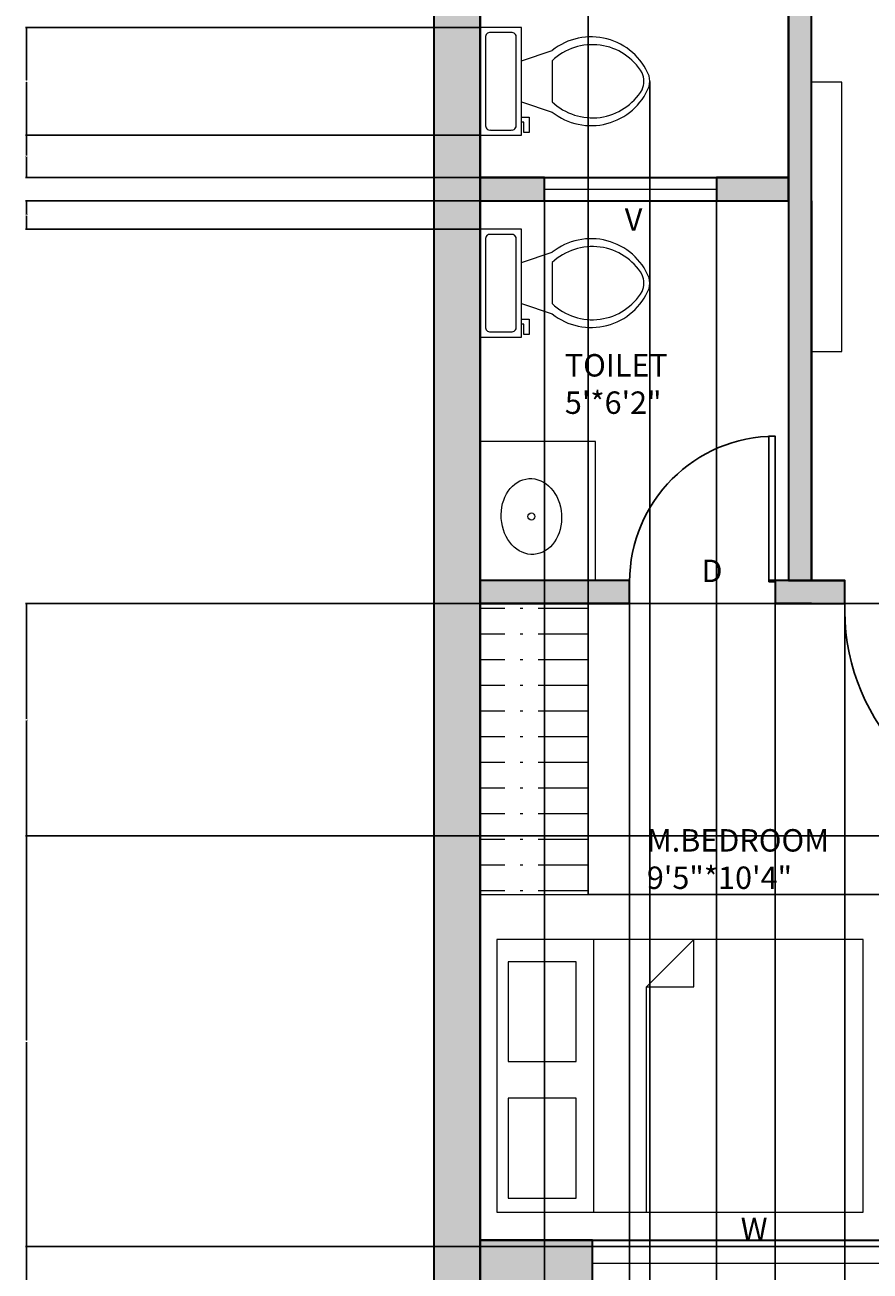
# Model space of a CAD drawing. Units: inches. Extents: x 2035 to 2384, y 1427 to 2020.
# Tile 2 of 7: x 2035 to 2200, y 1551 to 1794. Entities that reach past the tile are written whole.
import ezdxf

# ---------------------------------------------------------------- set-up
doc = ezdxf.new("R2010")
doc.units = ezdxf.units.IN
for name, color, linetype, lineweight in [('A-ANNO-DIMS', 2, 'Continuous', 18), ('A-ANNO-IDEN', 201, 'Continuous', 18), ('A-AREA-IDEN', 201, 'Continuous', 18), ('A-FLOR-CABN', 71, 'Continuous', 18), ('A-FLOR-CABN-PATT', 71, 'Continuous', 13), ('A-FLOR-FIXT', 9, 'Continuous', 18), ('A-WALL-PATT', 140, 'Continuous', 13), ('C-PROP', 7, 'Continuous', 25), ('DOOR', 52, 'Continuous', 25), ('FUR', 71, 'Continuous', 18), ('WALL', 140, 'Continuous', 35), ('WIN', 230, 'Continuous', 18)]:
    doc.layers.add(name, color=color, linetype=linetype, lineweight=lineweight)
doc.styles.get("Standard").update_dxf_attribs({"font": 'arial.ttf'})
doc.dimstyles.get("Standard").update_dxf_attribs({"dimtxt": 0.18, "dimasz": 0.18, "dimexe": 0.18, "dimexo": 0.0625, "dimgap": 0.09, "dimtad": 0, "dimtih": 1, "dimtoh": 1, "dimdec": 4, "dimzin": 0, "dimdsep": 46, "dimtxsty": 'Standard', "dimcen": 0.09, "dimadec": 0, "dimazin": 0, "dimtfac": 1, "dimtdec": 4, "dimtofl": 0, "dimtmove": 0, "dimatfit": 3, "dimfxl": 1, "dimtolj": 1, "dimtzin": 0, "dimarcsym": 0})

# ---------------------------------------------------------------- blocks, each defined once
blk = doc.blocks.new('*U2')
for p, q in [((0, 0), (0, -6)), ((40, 0), (40, -6))]:
    blk.add_line(p, q)
blk.add_lwpolyline([(0, 0), (0, 40), (1.75, 40), (1.75, 0)], close=True)
blk.add_arc((0, 0), 40, 0, 90)
blk = doc.blocks.new('*U4')
for p, q in [((9.5, -6), (9.5, -2)), ((-10, -8.5), (-8, -8.5)), ((-10, -9.5), (-10, -8.5)), ((-7, -9.5), (-10, -9.5)), ((-8, -8.5), (-8, -8)), ((-7, -8), (-7, -9.5)), ((-4, -8), (-6, -14)), ((4, -8), (6, -14)), ((4, -14), (-4, -14))]:
    blk.add_line(p, q)
blk.add_lwpolyline([(10.5, -8), (10.5, 0), (-10.5, 0), (-10.5, -8)], close=True)
for points in [[(-9.5, -2), (-9.5, -6)], [(8.5, -1), (-8.5, -1)], [(-8.5, -7), (8.5, -7)]]:
    blk.add_lwpolyline(points)
for centre, radius, start, end in [((-8.62, -1.88), 0.884, 81.8699, 188.1301), ((8.62, -1.88), 0.884, 351.8699, 98.1301), ((-8.62, -6.12), 0.884, 171.8699, 278.1301), ((8.62, -6.12), 0.884, 261.8699, 8.1301), ((3.52, -21.58), 12.17, 141.4691, 247.9714), ((4.2, -21.82), 11.33, 136.3677, 238.9468), ((-3.52, -21.58), 12.17, 292.0284, 38.5307), ((-4.2, -21.82), 11.33, 301.053, 43.6321), ((0, -27.88), 4, 245.7318, 294.2682), ((0, -29), 4, 254.8605, 285.1395)]:
    blk.add_arc(centre, radius, start, end)
blk = doc.blocks.new('BED-DOUBLE')
for p, q in [((18.86, 0), (18.86, 53.15)), ((38.37, 53.15), (29.1, 43.9)), ((38.37, 43.9), (38.37, 53.15)), ((29.1, 0), (29.1, 43.9)), ((29.1, 43.9), (38.37, 43.9))]:
    blk.add_line(p, q)
for points in [[(0, 0), (71.34, 0), (71.34, 53.15), (0, 53.15)], [(2.2, 29.34), (15.42, 29.34), (15.42, 48.81), (2.2, 48.81)], [(2.2, 2.74), (15.42, 2.74), (15.42, 22.21), (2.2, 22.21)]]:
    blk.add_lwpolyline(points, close=True)
blk = doc.blocks.new('BASIN-VANITY')
blk.add_lwpolyline([(0, 0), (22.45, 0), (22.45, 27.1), (0, 27.1)], close=True)
blk.add_circle((9.95, 12.48), 0.683)
blk.add_ellipse((9.95, 12.48), major_axis=(-0.5, 7.38), ratio=0.795414)
blk = doc.blocks.new('WIN-BEDROOM')
blk.add_line((0, 4.5), (63.76, 4.5))
blk.add_lwpolyline([(0, 9), (63.76, 9), (63.76, 0), (0, 0)], close=True)
blk = doc.blocks.new('*D28')
at = {"layer": 'A-ANNO-DIMS', "color": 0, "lineweight": -2, "transparency": 16777216}
for p, q in [((2345.69, 1555.63), (2035.17, 1555.63)), ((2035.35, 1555.45), (2035.35, 1531.25)), ((2035.35, 1506.68), (2035.35, 1530.88)), ((2323.05, 1506.5), (2035.17, 1506.5))]:
    blk.add_line(p, q, dxfattribs=at)
at = {"layer": 'A-ANNO-DIMS', "color": 0, "lineweight": 100, "transparency": 16777216}
for points in [[(2035.32, 1555.45), (2035.38, 1555.45), (2035.35, 1555.63)], [(2035.32, 1506.68), (2035.38, 1506.68), (2035.35, 1506.5)]]:
    blk.add_solid(points, dxfattribs=at)
at = {"layer": 'Defpoints', "color": 0, "lineweight": 100, "transparency": 16777216}
for p in [(2035.35, 1555.63), (2345.75, 1555.63), (2323.11, 1506.5)]:
    blk.add_point(p, dxfattribs=at)
at = {"layer": 'A-ANNO-DIMS', "color": 0, "transparency": 16777216, "insert": (2035.35, 1531.06), "char_height": 0.18, "attachment_point": 5}
blk.add_mtext('\\A1;49.14', dxfattribs=at)
blk = doc.blocks.new('*D29')
at = {"layer": 'A-ANNO-DIMS', "color": 0, "lineweight": -2, "transparency": 16777216}
for p, q in [((2309.69, 1635.63), (2035.17, 1635.63)), ((2035.35, 1635.45), (2035.35, 1595.81)), ((2035.35, 1555.81), (2035.35, 1595.45)), ((2309.69, 1555.63), (2035.17, 1555.63))]:
    blk.add_line(p, q, dxfattribs=at)
at = {"layer": 'A-ANNO-DIMS', "color": 0, "lineweight": 100, "transparency": 16777216}
for points in [[(2035.32, 1635.45), (2035.38, 1635.45), (2035.35, 1635.63)], [(2035.32, 1555.81), (2035.38, 1555.81), (2035.35, 1555.63)]]:
    blk.add_solid(points, dxfattribs=at)
at = {"layer": 'Defpoints', "color": 0, "lineweight": 100, "transparency": 16777216}
for p in [(2035.35, 1635.63), (2309.75, 1635.63), (2309.75, 1555.63)]:
    blk.add_point(p, dxfattribs=at)
at = {"layer": 'A-ANNO-DIMS', "color": 0, "transparency": 16777216, "insert": (2035.35, 1595.63), "char_height": 0.18, "attachment_point": 5}
blk.add_mtext('\\A1;80', dxfattribs=at)
blk = doc.blocks.new('*D30')
at = {"layer": 'A-ANNO-DIMS', "color": 0, "lineweight": -2, "transparency": 16777216}
for p, q in [((2309.69, 1680.88), (2035.17, 1680.88)), ((2035.35, 1680.7), (2035.35, 1658.44)), ((2035.35, 1635.81), (2035.35, 1658.07)), ((2309.69, 1635.63), (2035.17, 1635.63))]:
    blk.add_line(p, q, dxfattribs=at)
at = {"layer": 'A-ANNO-DIMS', "color": 0, "lineweight": 100, "transparency": 16777216}
for points in [[(2035.32, 1680.7), (2035.38, 1680.7), (2035.35, 1680.88)], [(2035.32, 1635.81), (2035.38, 1635.81), (2035.35, 1635.63)]]:
    blk.add_solid(points, dxfattribs=at)
at = {"layer": 'Defpoints', "color": 0, "lineweight": 100, "transparency": 16777216}
for p in [(2035.35, 1680.88), (2309.75, 1680.88), (2309.75, 1635.63)]:
    blk.add_point(p, dxfattribs=at)
at = {"layer": 'A-ANNO-DIMS', "color": 0, "transparency": 16777216, "insert": (2035.35, 1658.26), "char_height": 0.18, "attachment_point": 5}
blk.add_mtext('\\A1;45.25', dxfattribs=at)
blk = doc.blocks.new('*D34')
at = {"layer": 'A-ANNO-DIMS', "color": 0, "lineweight": -2, "transparency": 16777216}
for p, q in [((2194.77, 1680.82), (2194.77, 1427.17)), ((2234.77, 1680.82), (2234.77, 1427.17)), ((2194.95, 1427.35), (2214.55, 1427.35)), ((2234.59, 1427.35), (2214.99, 1427.35))]:
    blk.add_line(p, q, dxfattribs=at)
at = {"layer": 'A-ANNO-DIMS', "color": 0, "lineweight": 100, "transparency": 16777216}
for points in [[(2194.95, 1427.38), (2194.95, 1427.32), (2194.77, 1427.35)], [(2234.59, 1427.38), (2234.59, 1427.32), (2234.77, 1427.35)]]:
    blk.add_solid(points, dxfattribs=at)
at = {"layer": 'Defpoints', "color": 0, "lineweight": 100, "transparency": 16777216}
for p in [(2194.77, 1680.88), (2234.77, 1680.88), (2234.77, 1427.35)]:
    blk.add_point(p, dxfattribs=at)
at = {"layer": 'A-ANNO-DIMS', "color": 0, "transparency": 16777216, "insert": (2214.77, 1427.35), "char_height": 0.18, "attachment_point": 5}
blk.add_mtext('\\A1;40', dxfattribs=at)
blk = doc.blocks.new('*D37')
at = {"layer": 'A-ANNO-DIMS', "color": 0, "lineweight": -2, "transparency": 16777216}
for p, q in [((2152.83, 1680.82), (2152.83, 1427.17)), ((2181.2, 1680.82), (2181.2, 1427.17)), ((2153.01, 1427.35), (2166.62, 1427.35)), ((2181.02, 1427.35), (2167.41, 1427.35))]:
    blk.add_line(p, q, dxfattribs=at)
at = {"layer": 'A-ANNO-DIMS', "color": 0, "lineweight": 100, "transparency": 16777216}
for points in [[(2153.01, 1427.38), (2153.01, 1427.32), (2152.83, 1427.35)], [(2181.02, 1427.38), (2181.02, 1427.32), (2181.2, 1427.35)]]:
    blk.add_solid(points, dxfattribs=at)
at = {"layer": 'Defpoints', "color": 0, "lineweight": 100, "transparency": 16777216}
for p in [(2152.83, 1680.88), (2181.2, 1680.88), (2181.2, 1427.35)]:
    blk.add_point(p, dxfattribs=at)
at = {"layer": 'A-ANNO-DIMS', "color": 0, "transparency": 16777216, "insert": (2167.02, 1427.35), "char_height": 0.18, "attachment_point": 5}
blk.add_mtext('\\A1;28.37', dxfattribs=at)
blk = doc.blocks.new('*D39')
at = {"layer": 'A-ANNO-DIMS', "color": 0, "lineweight": -2, "transparency": 16777216}
for p, q in [((2136.25, 1759.32), (2136.25, 1427.17)), ((2169.78, 1759.32), (2169.78, 1427.17)), ((2136.43, 1427.35), (2152.62, 1427.35)), ((2169.6, 1427.35), (2153.41, 1427.35))]:
    blk.add_line(p, q, dxfattribs=at)
at = {"layer": 'A-ANNO-DIMS', "color": 0, "lineweight": 100, "transparency": 16777216}
for points in [[(2136.43, 1427.38), (2136.43, 1427.32), (2136.25, 1427.35)], [(2169.6, 1427.38), (2169.6, 1427.32), (2169.78, 1427.35)]]:
    blk.add_solid(points, dxfattribs=at)
at = {"layer": 'Defpoints', "color": 0, "lineweight": 100, "transparency": 16777216}
for p in [(2136.25, 1759.38), (2169.78, 1759.38), (2169.78, 1427.35)]:
    blk.add_point(p, dxfattribs=at)
at = {"layer": 'A-ANNO-DIMS', "color": 0, "transparency": 16777216, "insert": (2153.02, 1427.35), "char_height": 0.18, "attachment_point": 5}
blk.add_mtext('\\A1;33.52', dxfattribs=at)
blk = doc.blocks.new('*D50')
at = {"layer": 'A-ANNO-DIMS', "color": 0, "lineweight": -2, "transparency": 16777216}
for p, q in [((2156.75, 1782.6), (2156.75, 1427.17)), ((2123.75, 1772.1), (2123.75, 1427.17)), ((2123.93, 1427.35), (2140.03, 1427.35)), ((2156.57, 1427.35), (2140.47, 1427.35))]:
    blk.add_line(p, q, dxfattribs=at)
at = {"layer": 'A-ANNO-DIMS', "color": 0, "lineweight": 100, "transparency": 16777216}
for points in [[(2123.93, 1427.38), (2123.93, 1427.32), (2123.75, 1427.35)], [(2156.57, 1427.38), (2156.57, 1427.32), (2156.75, 1427.35)]]:
    blk.add_solid(points, dxfattribs=at)
at = {"layer": 'Defpoints', "color": 0, "lineweight": 100, "transparency": 16777216}
for p in [(2156.75, 1782.66), (2123.75, 1772.16), (2156.75, 1427.35)]:
    blk.add_point(p, dxfattribs=at)
at = {"layer": 'A-ANNO-DIMS', "color": 0, "transparency": 16777216, "insert": (2140.25, 1427.35), "char_height": 0.18, "attachment_point": 5}
blk.add_mtext('\\A1;33', dxfattribs=at)
blk = doc.blocks.new('*D51')
at = {"layer": 'A-ANNO-DIMS', "color": 0, "lineweight": -2, "transparency": 16777216}
for p, q in [((2123.69, 1793.16), (2035.17, 1793.16)), ((2035.35, 1792.98), (2035.35, 1782.84)), ((2035.35, 1772.34), (2035.35, 1782.48)), ((2123.69, 1772.16), (2035.17, 1772.16))]:
    blk.add_line(p, q, dxfattribs=at)
at = {"layer": 'A-ANNO-DIMS', "color": 0, "lineweight": 100, "transparency": 16777216}
for points in [[(2035.32, 1792.98), (2035.38, 1792.98), (2035.35, 1793.16)], [(2035.32, 1772.34), (2035.38, 1772.34), (2035.35, 1772.16)]]:
    blk.add_solid(points, dxfattribs=at)
at = {"layer": 'Defpoints', "color": 0, "lineweight": 100, "transparency": 16777216}
for p in [(2035.35, 1793.16), (2123.75, 1793.16), (2123.75, 1772.16)]:
    blk.add_point(p, dxfattribs=at)
at = {"layer": 'A-ANNO-DIMS', "color": 0, "transparency": 16777216, "insert": (2035.35, 1782.66), "char_height": 0.18, "attachment_point": 5}
blk.add_mtext('\\A1;21', dxfattribs=at)
blk = doc.blocks.new('*D52')
at = {"layer": 'A-ANNO-DIMS', "color": 0, "lineweight": -2, "transparency": 16777216}
for p, q in [((2123.69, 1772.16), (2035.17, 1772.16)), ((2035.35, 1771.98), (2035.35, 1768.2)), ((2035.35, 1764.06), (2035.35, 1767.84)), ((2123.69, 1763.88), (2035.17, 1763.88))]:
    blk.add_line(p, q, dxfattribs=at)
at = {"layer": 'A-ANNO-DIMS', "color": 0, "lineweight": 100, "transparency": 16777216}
for points in [[(2035.32, 1771.98), (2035.38, 1771.98), (2035.35, 1772.16)], [(2035.32, 1764.06), (2035.38, 1764.06), (2035.35, 1763.88)]]:
    blk.add_solid(points, dxfattribs=at)
at = {"layer": 'Defpoints', "color": 0, "lineweight": 100, "transparency": 16777216}
for p in [(2035.35, 1772.16), (2123.75, 1772.16), (2123.75, 1763.88)]:
    blk.add_point(p, dxfattribs=at)
at = {"layer": 'A-ANNO-DIMS', "color": 0, "transparency": 16777216, "insert": (2035.35, 1768.02), "char_height": 0.18, "attachment_point": 5}
blk.add_mtext('\\A1;8.277', dxfattribs=at)
blk = doc.blocks.new('*D53')
at = {"layer": 'A-ANNO-DIMS', "color": 0, "lineweight": -2, "transparency": 16777216}
for p, q in [((2123.69, 1759.38), (2035.17, 1759.38)), ((2035.35, 1759.2), (2035.35, 1756.79)), ((2035.35, 1754.01), (2035.35, 1756.43)), ((2123.69, 1753.83), (2035.17, 1753.83))]:
    blk.add_line(p, q, dxfattribs=at)
at = {"layer": 'A-ANNO-DIMS', "color": 0, "lineweight": 100, "transparency": 16777216}
for points in [[(2035.32, 1759.2), (2035.38, 1759.2), (2035.35, 1759.38)], [(2035.32, 1754.01), (2035.38, 1754.01), (2035.35, 1753.83)]]:
    blk.add_solid(points, dxfattribs=at)
at = {"layer": 'Defpoints', "color": 0, "lineweight": 100, "transparency": 16777216}
for p in [(2035.35, 1759.38), (2123.75, 1759.38), (2123.75, 1753.83)]:
    blk.add_point(p, dxfattribs=at)
at = {"layer": 'A-ANNO-DIMS', "color": 0, "transparency": 16777216, "insert": (2035.35, 1756.61), "char_height": 0.18, "attachment_point": 5}
blk.add_mtext('\\A1;5.55', dxfattribs=at)
blk = doc.blocks.new('*D62')
at = {"layer": 'A-ANNO-DIMS', "color": 0, "lineweight": -2, "transparency": 16777216}
for p, q in [((2123.75, 1624.27), (2123.75, 2009.96)), ((2123.93, 2009.78), (2133.8, 2009.78)), ((2144.6, 2009.78), (2134.73, 2009.78)), ((2144.78, 1624.27), (2144.78, 2009.96))]:
    blk.add_line(p, q, dxfattribs=at)
at = {"layer": 'A-ANNO-DIMS', "color": 0, "lineweight": 100, "transparency": 16777216}
for points in [[(2123.93, 2009.81), (2123.93, 2009.75), (2123.75, 2009.78)], [(2144.6, 2009.81), (2144.6, 2009.75), (2144.78, 2009.78)]]:
    blk.add_solid(points, dxfattribs=at)
at = {"layer": 'Defpoints', "color": 0, "lineweight": 100, "transparency": 16777216}
for p in [(2144.78, 2009.78), (2123.75, 1624.2), (2144.78, 1624.2)]:
    blk.add_point(p, dxfattribs=at)
at = {"layer": 'A-ANNO-DIMS', "color": 0, "transparency": 16777216, "insert": (2134.27, 2009.78), "char_height": 0.18, "attachment_point": 5}
blk.add_mtext('\\A1;21.028', dxfattribs=at)
blk = doc.blocks.new('*D63')
at = {"layer": 'A-ANNO-DIMS', "color": 0, "lineweight": -2, "transparency": 16777216}
for p, q in [((2144.84, 1680.88), (2383.33, 1680.88)), ((2383.15, 1680.7), (2383.15, 1652.72)), ((2383.15, 1624.38), (2383.15, 1652.36)), ((2144.84, 1624.2), (2383.33, 1624.2))]:
    blk.add_line(p, q, dxfattribs=at)
at = {"layer": 'A-ANNO-DIMS', "color": 0, "lineweight": 100, "transparency": 16777216}
for points in [[(2383.12, 1680.7), (2383.18, 1680.7), (2383.15, 1680.88)], [(2383.12, 1624.38), (2383.18, 1624.38), (2383.15, 1624.2)]]:
    blk.add_solid(points, dxfattribs=at)
at = {"layer": 'Defpoints', "color": 0, "lineweight": 100, "transparency": 16777216}
for p in [(2144.78, 1680.88), (2383.15, 1680.88), (2144.78, 1624.2)]:
    blk.add_point(p, dxfattribs=at)
at = {"layer": 'A-ANNO-DIMS', "color": 0, "transparency": 16777216, "insert": (2383.15, 1652.54), "char_height": 0.18, "attachment_point": 5}
blk.add_mtext('\\A1;56.68', dxfattribs=at)

msp = doc.modelspace()

# ---------------------------------------------------------------- hatches: boundary and pattern name
at = {"layer": 'A-FLOR-CABN-PATT'}
h = msp.add_hatch(dxfattribs=at)
h.set_pattern_fill('ACAD_ISO04W100', color=256)
h.paths.add_polyline_path([(2144.7806, 1680.8816), (2123.7529, 1680.8816), (2123.7529, 1624.204), (2144.7806, 1624.204)])
at = {"layer": 'A-WALL-PATT'}
h = msp.add_hatch(color=256, dxfattribs=at)
h.dxf.hatch_style = 1
h.paths.add_polyline_path([(2145.6215, 1981.3816), (2123.7529, 1981.3816), (2123.7529, 1972.3816), (2145.6215, 1972.3816)])
h.paths.add_polyline_path([(2354.7529, 1981.3816), (2209.3767, 1981.3816), (2209.3767, 1972.3816), (2354.7529, 1972.3816)])
h.paths.add_polyline_path([(2123.7529, 1981.3816), (2114.7529, 1981.3816), (2114.7529, 1505.8816), (2123.7529, 1505.8816)])
h.paths.add_polyline_path([(2248.2529, 1928.1316), (2243.7529, 1928.1316), (2243.7529, 1840.3816), (2248.2529, 1840.3816)])
h.paths.add_polyline_path([(2297.0514, 1930.3816), (2284.6994, 1930.3816), (2284.6994, 1925.8816), (2297.0514, 1925.8816)])
h.paths.add_polyline_path([(2345.7529, 1930.3816), (2333.1098, 1930.3816), (2333.1098, 1925.8816), (2345.7529, 1925.8816)])
h.paths.add_polyline_path([(2354.7529, 1972.3816), (2345.7529, 1972.3816), (2345.7529, 1501.3816), (2354.7529, 1501.3816)])
h.paths.add_polyline_path([(2188.2529, 1835.8816), (2183.7529, 1835.8816), (2183.7529, 1831.3677), (2184.207, 1831.3677), (2188.2529, 1831.3677)])
h.paths.add_polyline_path([(2188.2529, 1804.3949), (2184.207, 1804.3949), (2183.7529, 1804.3949), (2183.7529, 1685.3816), (2188.2529, 1685.3816)])
h.paths.add_polyline_path([(2273.5087, 1840.3816), (2241.0146, 1840.3816), (2241.0146, 1835.8816), (2273.5087, 1835.8816)])
h.paths.add_polyline_path([(2345.7529, 1840.3816), (2310.4577, 1840.3816), (2310.4577, 1835.8816), (2345.7529, 1835.8816)])
h.paths.add_polyline_path([(2161.9064, 1524.4315), (2196.2972, 1524.4315), (2196.2972, 1533.4306), (2161.9064, 1533.4306)], flags=9)
h.paths.add_polyline_path([(2279.3058, 1589.7515), (2308.9483, 1589.7515), (2308.9483, 1598.7506), (2279.3058, 1598.7506)], flags=9)
h.paths.add_polyline_path([(2242.9684, 1662.1655), (2279.0513, 1662.1655), (2279.0513, 1671.1647), (2242.9684, 1671.1647)], flags=9)
h.paths.add_polyline_path([(2154.6483, 1622.8242), (2195.1309, 1622.8242), (2195.1309, 1639.1195), (2154.6483, 1639.1195)], flags=9)
h.paths.add_polyline_path([(2138.8708, 1715.378), (2162.5199, 1715.378), (2162.5199, 1731.6734), (2138.8708, 1731.6734)], flags=9)
h.paths.add_polyline_path([(2135.5598, 1791.707), (2165.1993, 1791.707), (2165.1993, 1808.0024), (2135.5598, 1808.0024)], flags=9)
h.paths.add_polyline_path([(2245.1071, 1740.4502), (2279.0303, 1740.4502), (2279.0303, 1756.7455), (2245.1071, 1756.7455)], flags=9)
h.paths.add_polyline_path([(2284.7312, 1866.5552), (2313.6916, 1866.5552), (2313.6916, 1890.2034), (2284.7312, 1890.2034)], flags=9)
h.paths.add_polyline_path([(2139.9071, 1874.6496), (2173.8303, 1874.6496), (2173.8303, 1890.9449), (2139.9071, 1890.9449)], flags=9)
h = msp.add_hatch(color=256, dxfattribs=at)
h.dxf.hatch_style = 1
h.paths.add_polyline_path([(2236.7529, 1556.8816), (2209.3767, 1556.8816), (2209.3767, 1547.8816), (2236.7529, 1547.8816)])
h.paths.add_polyline_path([(2241.2529, 1680.8816), (2236.7529, 1680.8816), (2236.7529, 1547.8816), (2241.2529, 1547.8816)])
h.paths.add_polyline_path([(2241.2529, 1505.8816), (2114.7529, 1505.8816), (2114.7529, 1501.3816), (2241.2529, 1501.3816)])
h.paths.add_polyline_path([(2242.179, 1683.1823), (2242.179, 1685.3816), (2234.769, 1685.3816), (2234.769, 1680.8816), (2242.179, 1680.8816)])
h.paths.add_polyline_path([(2286.8795, 1685.3816), (2272.8549, 1685.3816), (2272.8549, 1683.1823), (2272.8549, 1680.8816), (2286.8795, 1680.8816)])
h.paths.add_polyline_path([(2345.7529, 1685.3816), (2329.513, 1685.3816), (2329.513, 1680.8816), (2345.7529, 1680.8816)])
h.paths.add_polyline_path([(2279.3058, 1589.7515), (2308.9483, 1589.7515), (2308.9483, 1598.7506), (2279.3058, 1598.7506)], flags=9)
h.paths.add_polyline_path([(2242.9684, 1662.1655), (2279.0513, 1662.1655), (2279.0513, 1671.1647), (2242.9684, 1671.1647)], flags=9)
h.paths.add_polyline_path([(2154.6483, 1622.8242), (2195.1309, 1622.8242), (2195.1309, 1639.1195), (2154.6483, 1639.1195)], flags=9)
h.paths.add_polyline_path([(2138.8708, 1715.378), (2162.5199, 1715.378), (2162.5199, 1731.6734), (2138.8708, 1731.6734)], flags=9)
h.paths.add_polyline_path([(2135.5598, 1791.707), (2165.1993, 1791.707), (2165.1993, 1808.0024), (2135.5598, 1808.0024)], flags=9)
h.paths.add_polyline_path([(2245.1071, 1740.4502), (2279.0303, 1740.4502), (2279.0303, 1756.7455), (2245.1071, 1756.7455)], flags=9)
h.paths.add_polyline_path([(2284.7312, 1866.5552), (2313.6916, 1866.5552), (2313.6916, 1890.2034), (2284.7312, 1890.2034)], flags=9)
h.paths.add_polyline_path([(2284.6985, 1943.1527), (2309.7208, 1943.1527), (2309.7208, 1959.448), (2284.6985, 1959.448)], flags=9)
h.paths.add_polyline_path([(2139.9071, 1874.6496), (2173.8303, 1874.6496), (2173.8303, 1890.9449), (2139.9071, 1890.9449)], flags=9)
h = msp.add_hatch(color=256, dxfattribs=at)
h.dxf.hatch_style = 1
h.paths.add_polyline_path([(2201.0146, 1840.3816), (2123.7529, 1840.3816), (2123.7529, 1835.8816), (2201.0146, 1835.8816)])
h.paths.add_polyline_path([(2136.2543, 1763.8816), (2123.7529, 1763.8816), (2123.7529, 1759.3816), (2136.2543, 1759.3816)])
h.paths.add_polyline_path([(2183.7529, 1763.8816), (2169.7769, 1763.8816), (2169.7769, 1759.3816), (2183.7529, 1759.3816)])
h.paths.add_polyline_path([(2152.8338, 1685.1369), (2152.8338, 1685.3816), (2123.7529, 1685.3816), (2123.7529, 1680.8816), (2152.8338, 1680.8816)])
h.paths.add_polyline_path([(2194.769, 1685.3816), (2181.2028, 1685.3816), (2181.2028, 1685.1369), (2181.2028, 1680.8816), (2194.769, 1680.8816)])
h.paths.add_polyline_path([(2145.6215, 1556.8816), (2123.7529, 1556.8816), (2123.7529, 1547.8816), (2145.6215, 1547.8816)])
h.paths.add_polyline_path([(2161.9064, 1524.4315), (2196.2972, 1524.4315), (2196.2972, 1533.4306), (2161.9064, 1533.4306)], flags=9)
h.paths.add_polyline_path([(2279.3058, 1589.7515), (2308.9483, 1589.7515), (2308.9483, 1598.7506), (2279.3058, 1598.7506)], flags=9)
h.paths.add_polyline_path([(2242.9684, 1662.1655), (2279.0513, 1662.1655), (2279.0513, 1671.1647), (2242.9684, 1671.1647)], flags=9)
h.paths.add_polyline_path([(2154.6483, 1622.8242), (2195.1309, 1622.8242), (2195.1309, 1639.1195), (2154.6483, 1639.1195)], flags=9)
h.paths.add_polyline_path([(2138.8708, 1715.378), (2162.5199, 1715.378), (2162.5199, 1731.6734), (2138.8708, 1731.6734)], flags=9)
h.paths.add_polyline_path([(2135.5598, 1791.707), (2165.1993, 1791.707), (2165.1993, 1808.0024), (2135.5598, 1808.0024)], flags=9)
h.paths.add_polyline_path([(2245.1071, 1740.4502), (2279.0303, 1740.4502), (2279.0303, 1756.7455), (2245.1071, 1756.7455)], flags=9)
h.paths.add_polyline_path([(2284.7312, 1866.5552), (2313.6916, 1866.5552), (2313.6916, 1890.2034), (2284.7312, 1890.2034)], flags=9)
h.paths.add_polyline_path([(2284.6985, 1943.1527), (2309.7208, 1943.1527), (2309.7208, 1959.448), (2284.6985, 1959.448)], flags=9)
h.paths.add_polyline_path([(2139.9071, 1874.6496), (2173.8303, 1874.6496), (2173.8303, 1890.9449), (2139.9071, 1890.9449)], flags=9)

# ---------------------------------------------------------------- linework, layer by layer
at = {"layer": 'A-FLOR-CABN'}
msp.add_lwpolyline([(2123.7529, 1624.204), (2144.7806, 1624.204), (2144.7806, 1680.8816), (2123.7529, 1680.8816)], close=True, dxfattribs=at)
at = {"layer": 'C-PROP'}
msp.add_line((2114.7529, 1501.3816), (2114.7529, 1981.3816), dxfattribs=at)
msp.add_lwpolyline([(2114.7529, 1981.3816), (2354.7529, 1981.3816), (2354.7529, 1501.3816), (2114.7529, 1501.3816)], close=True, dxfattribs=at)
at = {"layer": 'FUR'}
msp.add_lwpolyline([(2188.2529, 1729.9932), (2194.1963, 1729.9932), (2194.1963, 1782.4965), (2188.2529, 1782.4965)], close=True, dxfattribs=at)
at = {"layer": 'WALL'}
for p, q in [((2123.7529, 1835.8816), (2123.7529, 1763.8816)), ((2183.7529, 1763.8816), (2183.7529, 1804.3987)), ((2188.2529, 1759.3816), (2188.2529, 1804.3949)), ((2123.7529, 1763.8816), (2183.7529, 1763.8816)), ((2123.7529, 1759.3816), (2183.7529, 1759.3816)), ((2183.7529, 1759.3816), (2183.7529, 1685.3816)), ((2188.2529, 1759.3816), (2188.2529, 1685.3816)), ((2152.8348, 1685.3816), (2123.7529, 1685.3816)), ((2183.7529, 1685.3816), (2179.9617, 1685.3816)), ((2188.2529, 1685.3816), (2194.769, 1685.3816)), ((2123.7529, 1680.8816), (2123.7529, 1556.8816)), ((2152.8338, 1680.8816), (2123.7529, 1680.8816)), ((2188.2529, 1680.8816), (2181.2028, 1680.8816)), ((2188.2529, 1680.8816), (2194.769, 1680.8816)), ((2123.7529, 1556.8816), (2236.7529, 1556.8816))]:
    msp.add_line(p, q, dxfattribs=at)
for points in [[(2114.7529, 1981.3816), (2123.7529, 1981.3816), (2123.7529, 1505.8816), (2114.7529, 1505.8816)], [(2188.2529, 1804.3949), (2183.7529, 1804.3949), (2183.7529, 1685.3816), (2188.2529, 1685.3816)], [(2123.7529, 1759.3816), (2136.2543, 1759.3816), (2136.2543, 1763.8816), (2123.7529, 1763.8816)], [(2183.7529, 1763.8816), (2169.7769, 1763.8816), (2169.7769, 1759.3816), (2183.7529, 1759.3816)], [(2152.8338, 1685.3816), (2123.7529, 1685.3816), (2123.7529, 1680.8816), (2152.8338, 1680.8816)], [(2181.2028, 1680.8816), (2194.769, 1680.8816), (2194.769, 1685.3816), (2181.2028, 1685.3816)], [(2145.6215, 1556.8816), (2123.7529, 1556.8816), (2123.7529, 1547.8816), (2145.6215, 1547.8816)]]:
    msp.add_lwpolyline(points, close=True, dxfattribs=at)
msp.add_lwpolyline([(2241.2529, 1552.3816), (2241.2529, 1505.8816), (2123.7529, 1505.8816), (2123.7529, 1972.3816), (2345.7529, 1972.3816), (2345.7529, 1503.6316), (2323.1125, 1503.6316)], dxfattribs=at)
at = {"layer": 'WIN'}
msp.add_line((2136.2543, 1761.6316), (2169.7769, 1761.6316), dxfattribs=at)
msp.add_lwpolyline([(2136.2543, 1759.3816), (2169.7769, 1759.3816), (2169.7769, 1763.8816), (2136.2543, 1763.8816)], close=True, dxfattribs=at)

# ---------------------------------------------------------------- block references
at = {"layer": 'A-FLOR-FIXT', "rotation": 90}
for p in [(2123.7529, 1782.6583), (2123.7529, 1743.3321)]:
    msp.add_blockref('*U4', p, dxfattribs=at)
at = {"layer": 'A-FLOR-FIXT'}
msp.add_blockref('BASIN-VANITY', (2123.7529, 1685.3816), dxfattribs=at)
at = {"layer": 'DOOR', "xscale": -0.7092263827442089, "yscale": 0.7092263827442089, "zscale": 0.7092263827442089}
msp.add_blockref('*U2', (2181.2028, 1685.1369), dxfattribs=at)
at = {"layer": 'DOOR', "rotation": 180}
msp.add_blockref('*U2', (2234.769, 1679.3816), dxfattribs=at)
at = {"layer": 'FUR'}
msp.add_blockref('BED-DOUBLE', (2126.9898, 1562.3153), dxfattribs=at)
at = {"layer": 'WIN'}
msp.add_blockref('WIN-BEDROOM', (2145.6215, 1547.8816), dxfattribs=at)

# ---------------------------------------------------------------- texts
at = {"layer": 'A-ANNO-IDEN', "char_height": 4.367, "attachment_point": 1}
for s, insert in [('V', (2151.8859, 1757.9003)), ('D', (2166.8287, 1689.4508)), ('W', (2174.4677, 1561.2486))]:
    msp.add_mtext_dynamic_manual_height_columns(s, width=88.030619, gutter_width=21.835, heights=[0], dxfattribs=dict(at, insert=insert))
at = {"layer": 'A-AREA-IDEN', "char_height": 4.367, "attachment_point": 1}
for s, insert in [('TOILET\\P5\'*6\'2"', (2140.2157, 1729.5033)), ('M.BEDROOM\\P9\'5"*10\'4"', (2156.1928, 1636.9494))]:
    msp.add_mtext_dynamic_manual_height_columns(s, width=88.030619, gutter_width=21.835, heights=[0], dxfattribs=dict(at, insert=insert))

# ---------------------------------------------------------------- dimensions: what is measured, and where the dimension line sits
at = {"layer": 'A-ANNO-DIMS'}
for base, p1, p2, override, picture, middle in [((2144.7806, 2009.7816), (2123.7529, 1624.204), (2144.7806, 1624.204), {"dimdec": 3, "dimlfac": 1, "dimrnd": 0, "dimzin": 0, "dimdsep": 46, "dimlunit": 2}, '*D62', (2134.2668, 2009.7816)), ((2156.7529, 1427.3483), (2123.7529, 1772.1583), (2156.7529, 1782.6583), {"dimdec": 0, "dimlfac": 1, "dimrnd": 0, "dimzin": 0, "dimdsep": 46, "dimlunit": 2}, '*D50', (2140.2529, 1427.3483)), ((2169.7769, 1427.3483), (2136.2543, 1759.3816), (2169.7769, 1759.3816), {"dimdec": 2, "dimlfac": 1, "dimrnd": 0, "dimzin": 0, "dimdsep": 46, "dimlunit": 2}, '*D39', (2153.0156, 1427.3483)), ((2181.2028, 1427.3483), (2152.8338, 1680.8816), (2181.2028, 1680.8816), {"dimdec": 2, "dimlfac": 1, "dimrnd": 0, "dimzin": 0, "dimdsep": 46, "dimlunit": 2}, '*D37', (2167.0183, 1427.3483)), ((2234.769, 1427.3483), (2194.769, 1680.8816), (2234.769, 1680.8816), {"dimdec": 0, "dimlfac": 1, "dimrnd": 0, "dimzin": 0, "dimdsep": 46, "dimlunit": 2}, '*D34', (2214.769, 1427.3483))]:
    dim = msp.add_linear_dim(base=base, p1=p1, p2=p2, dimstyle='Standard', override=override, dxfattribs=at)
    dim.commit()
    dim.dimension.update_dxf_attribs({"geometry": picture, "text_midpoint": middle})
for base, p1, p2, override, picture, middle in [((2035.3529, 1793.1583), (2123.7529, 1772.1583), (2123.7529, 1793.1583), {"dimdec": 0, "dimlfac": 1, "dimrnd": 0, "dimzin": 0, "dimdsep": 46, "dimlunit": 2}, '*D51', (2035.3529, 1782.6583)), ((2035.3529, 1772.1583), (2123.7529, 1763.8816), (2123.7529, 1772.1583), {"dimdec": 3, "dimlfac": 1, "dimrnd": 0, "dimzin": 0, "dimdsep": 46, "dimlunit": 2}, '*D52', (2035.3529, 1768.0199)), ((2035.3529, 1759.3816), (2123.7529, 1753.8321), (2123.7529, 1759.3816), {"dimdec": 2, "dimlfac": 1, "dimrnd": 0, "dimzin": 0, "dimdsep": 46, "dimlunit": 2}, '*D53', (2035.3529, 1756.6068)), ((2035.3529, 1680.8816), (2309.7529, 1635.6316), (2309.7529, 1680.8816), {"dimdec": 2, "dimlfac": 1, "dimrnd": 0, "dimzin": 0, "dimdsep": 46, "dimlunit": 2}, '*D30', (2035.3529, 1658.2566)), ((2383.1529, 1680.8816), (2144.7806, 1624.204), (2144.7806, 1680.8816), {"dimdec": 2, "dimlfac": 1, "dimrnd": 0, "dimzin": 0, "dimdsep": 46, "dimlunit": 2}, '*D63', (2383.1529, 1652.5428)), ((2035.3529, 1635.6316), (2309.7529, 1555.6316), (2309.7529, 1635.6316), {"dimdec": 0, "dimlfac": 1, "dimrnd": 0, "dimzin": 0, "dimdsep": 46, "dimlunit": 2}, '*D29', (2035.3529, 1595.6316)), ((2035.3529, 1555.6316), (2323.1125, 1506.4959), (2345.7529, 1555.6316), {"dimdec": 2, "dimlfac": 1, "dimrnd": 0, "dimzin": 0, "dimdsep": 46, "dimlunit": 2}, '*D28', (2035.3529, 1531.0637))]:
    dim = msp.add_linear_dim(base=base, p1=p1, p2=p2, angle=90, dimstyle='Standard', override=override, dxfattribs=at)
    dim.commit()
    dim.dimension.update_dxf_attribs({"geometry": picture, "text_midpoint": middle})

doc.saveas('drawing.dxf')
